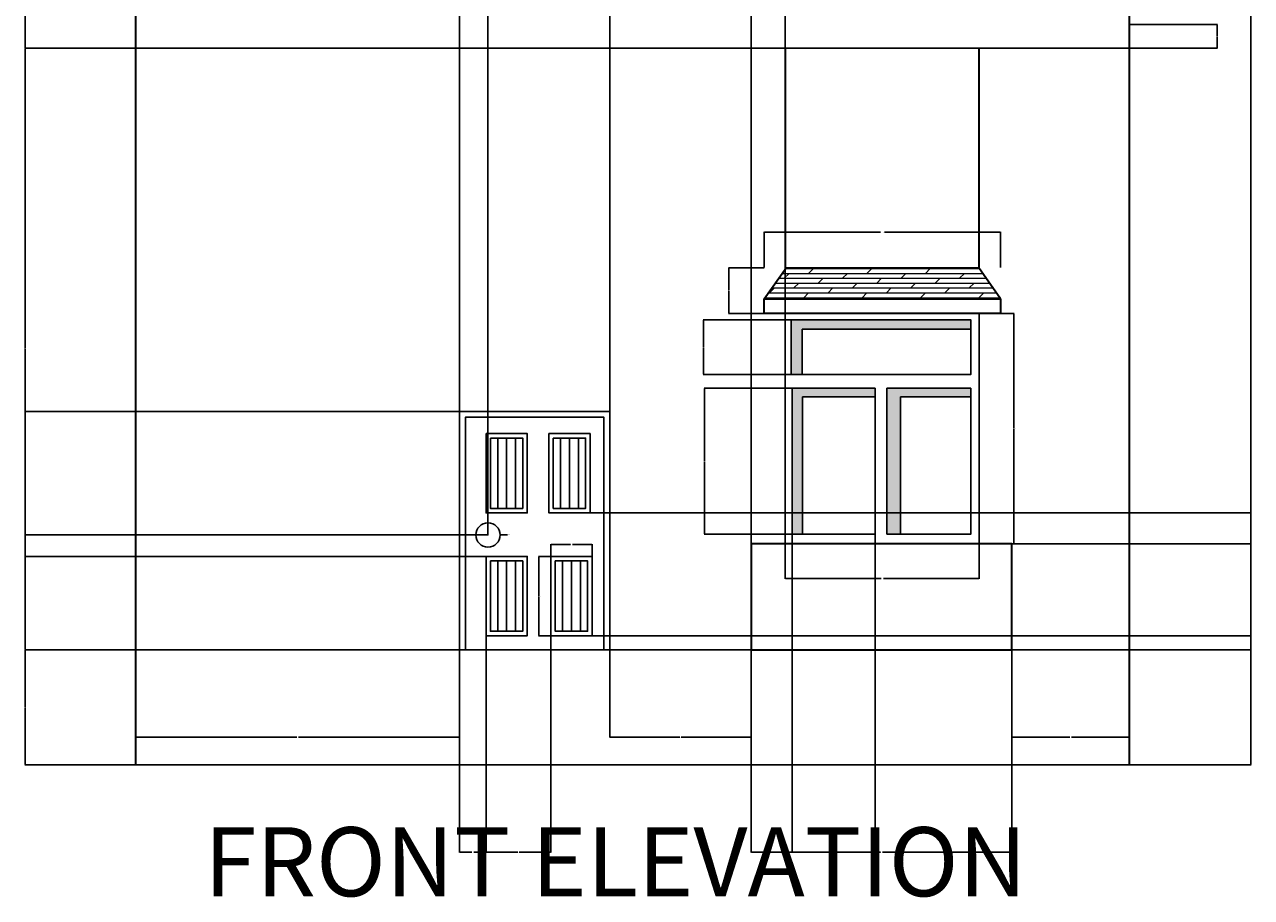
# Model space of a CAD drawing. Units: inches. Extents: x 1722 to 2362, y 1673 to 2617.
# Tile 1 of 2: x 1722 to 2362, y 1673 to 2129. Entities that reach past the tile are written whole.
import ezdxf

# ---------------------------------------------------------------- set-up
doc = ezdxf.new("R2010")
doc.units = ezdxf.units.IN
for name, color, linetype, lineweight in [('A-ANNO-DIMS', 2, 'Continuous', 18), ('A-ANNO-TEXT', 7, 'Continuous', 25), ('A-DOOR', 3, 'Continuous', 25), ('A-FLOR', 7, 'Continuous', 30), ('A-GLAZ', 4, 'Continuous', 25), ('A-GLAZ-PATT', 8, 'Continuous', 13), ('A-ROOF', 7, 'Continuous', 35), ('A-ROOF-PATT', 8, 'Continuous', 13), ('A-WALL', 7, 'Continuous', 35)]:
    doc.layers.add(name, color=color, linetype=linetype, lineweight=lineweight)
doc.styles.get("Standard").update_dxf_attribs({"font": 'arial.ttf'})
doc.dimstyles.get("Standard").update_dxf_attribs({"dimtxt": 0.18, "dimasz": 0.18, "dimexe": 0.18, "dimexo": 0.0625, "dimgap": 0.09, "dimtad": 0, "dimtih": 1, "dimtoh": 1, "dimdec": 4, "dimzin": 0, "dimdsep": 46, "dimtxsty": 'Standard', "dimcen": 0.09, "dimadec": 0, "dimazin": 0, "dimtfac": 1, "dimtdec": 4, "dimtofl": 0, "dimtmove": 0, "dimatfit": 3, "dimfxl": 1, "dimtolj": 1, "dimtzin": 0, "dimarcsym": 0})

# ---------------------------------------------------------------- blocks, each defined once
blk = doc.blocks.new('DOOR-PANEL-FLUTED')
for p, q in [((6.1, 39.03), (6.1, 2.33)), ((10.76, 39.03), (10.76, 2.33)), ((15.43, 39.03), (15.43, 2.33))]:
    blk.add_line(p, q)
for points in [[(0, 41.36), (21.52, 41.36), (21.52, 0), (0, 0)], [(2.33, 39.03), (19.19, 39.03), (19.19, 2.33), (2.33, 2.33)]]:
    blk.add_lwpolyline(points, close=True)
blk = doc.blocks.new('WIN-TWIN-TRANSOM')
for p, q in [((101.33, 120.15), (0, 120.15)), ((0, 120.15), (0, 0)), ((101.33, 0), (101.33, 120.15)), ((8.83, 88.28), (8.83, 111.99)), ((8.83, 111.99), (96.81, 111.99)), ((47.03, 81.23), (47.03, 5.04)), ((53.04, 81.23), (53.04, 5.04)), ((9.1, 76.71), (9.1, 5.04)), ((9.1, 76.71), (47.03, 76.71)), ((60.23, 76.71), (60.23, 5.04)), ((60.23, 76.71), (96.88, 76.71))]:
    blk.add_line(p, q)
blk.add_lwpolyline([(3.1, 116.89), (96.81, 116.89), (96.81, 88.28), (3.1, 88.28)], close=True)
for points in [[(47.03, 5.04), (3.67, 5.04), (3.67, 81.23), (47.03, 81.23)], [(53.04, 81.23), (96.88, 81.23), (96.88, 5.04), (53.04, 5.04)]]:
    blk.add_lwpolyline(points)
blk = doc.blocks.new('WIN-HOOD')
for p, q in [((0, 7.63), (11.4, 23.91)), ((11.4, 23.91), (111.91, 23.91)), ((123.31, 7.63), (111.91, 23.91)), ((0, 7.63), (123.31, 7.63)), ((0, 0), (0, 7.63)), ((123.31, 7.63), (123.31, 0)), ((123.31, 0), (0, 0))]:
    blk.add_line(p, q)
blk = doc.blocks.new('*D4')
at = {"layer": 'A-ANNO-DIMS', "color": 0, "lineweight": -2, "transparency": 16777216}
for p, q in [((1996.55, 1851.29), (1990.23, 1851.29)), ((1990.41, 1851.11), (1990.41, 1830.79)), ((1990.41, 1810.11), (1990.41, 1830.43)), ((1996.55, 1809.93), (1990.23, 1809.93))]:
    blk.add_line(p, q, dxfattribs=at)
at = {"layer": 'A-ANNO-DIMS', "color": 0, "transparency": 16777216}
for points in [[(1990.38, 1851.11), (1990.44, 1851.11), (1990.41, 1851.29)], [(1990.38, 1810.11), (1990.44, 1810.11), (1990.41, 1809.93)]]:
    blk.add_solid(points, dxfattribs=at)
at = {"layer": 'Defpoints', "color": 0, "transparency": 16777216}
for p in [(1990.41, 1851.29), (1996.61, 1851.29), (1996.61, 1809.93)]:
    blk.add_point(p, dxfattribs=at)
at = {"layer": 'A-ANNO-DIMS', "color": 0, "transparency": 16777216, "insert": (1990.41, 1830.61), "char_height": 0.18, "attachment_point": 5}
blk.add_mtext('\\A1;PANEL 41 TYP.', dxfattribs=at)
blk = doc.blocks.new('*D5')
at = {"layer": 'A-ANNO-DIMS', "color": 0, "lineweight": -2, "transparency": 16777216}
for p, q in [((1996.61, 1851.35), (1996.61, 1857.67)), ((1996.79, 1857.49), (2006.84, 1857.49)), ((2017.95, 1857.49), (2007.9, 1857.49)), ((2018.13, 1851.35), (2018.13, 1857.67))]:
    blk.add_line(p, q, dxfattribs=at)
at = {"layer": 'A-ANNO-DIMS', "color": 0, "transparency": 16777216}
for points in [[(1996.79, 1857.52), (1996.79, 1857.46), (1996.61, 1857.49)], [(2017.95, 1857.52), (2017.95, 1857.46), (2018.13, 1857.49)]]:
    blk.add_solid(points, dxfattribs=at)
at = {"layer": 'Defpoints', "color": 0, "transparency": 16777216}
for p in [(2018.13, 1857.49), (1996.61, 1851.29), (2018.13, 1851.29)]:
    blk.add_point(p, dxfattribs=at)
at = {"layer": 'A-ANNO-DIMS', "color": 0, "transparency": 16777216, "insert": (2007.37, 1857.49), "char_height": 0.18, "attachment_point": 5}
blk.add_mtext('\\A1;22 TYP.', dxfattribs=at)
blk = doc.blocks.new('*D6')
at = {"layer": 'A-ANNO-DIMS', "color": 0, "lineweight": -2, "transparency": 16777216}
for p, q in [((2220.22, 1977.99), (2238.36, 1977.99)), ((2238.18, 1977.81), (2238.18, 1918.1)), ((2238.18, 1858.02), (2238.18, 1917.74)), ((2220.22, 1857.84), (2238.36, 1857.84))]:
    blk.add_line(p, q, dxfattribs=at)
at = {"layer": 'A-ANNO-DIMS', "color": 0, "transparency": 16777216}
for points in [[(2238.15, 1977.81), (2238.21, 1977.81), (2238.18, 1977.99)], [(2238.15, 1858.02), (2238.21, 1858.02), (2238.18, 1857.84)]]:
    blk.add_solid(points, dxfattribs=at)
at = {"layer": 'Defpoints', "color": 0, "transparency": 16777216}
for p in [(2220.16, 1977.99), (2238.18, 1977.99), (2220.16, 1857.84)]:
    blk.add_point(p, dxfattribs=at)
at = {"layer": 'A-ANNO-DIMS', "color": 0, "transparency": 16777216, "insert": (2238.18, 1917.92), "char_height": 0.18, "attachment_point": 5}
blk.add_mtext('\\A1;WINDOW 120 TYP.', dxfattribs=at)
blk = doc.blocks.new('*D7')
at = {"layer": 'A-ANNO-DIMS', "color": 0, "lineweight": -2, "transparency": 16777216}
for p, q in [((2118.83, 1857.78), (2118.83, 1839.64)), ((2220.16, 1857.78), (2220.16, 1839.64)), ((2119.01, 1839.82), (2168.9, 1839.82)), ((2219.98, 1839.82), (2170.08, 1839.82))]:
    blk.add_line(p, q, dxfattribs=at)
at = {"layer": 'A-ANNO-DIMS', "color": 0, "transparency": 16777216}
for points in [[(2119.01, 1839.85), (2119.01, 1839.79), (2118.83, 1839.82)], [(2219.98, 1839.85), (2219.98, 1839.79), (2220.16, 1839.82)]]:
    blk.add_solid(points, dxfattribs=at)
at = {"layer": 'Defpoints', "color": 0, "transparency": 16777216}
for p in [(2118.83, 1857.84), (2220.16, 1857.84), (2220.16, 1839.82)]:
    blk.add_point(p, dxfattribs=at)
at = {"layer": 'A-ANNO-DIMS', "color": 0, "transparency": 16777216, "insert": (2169.49, 1839.82), "char_height": 0.18, "attachment_point": 5}
blk.add_mtext('\\A1;101 TYP.', dxfattribs=at)
blk = doc.blocks.new('*D8')
at = {"layer": 'A-ANNO-DIMS', "color": 0, "lineweight": -2, "transparency": 16777216}
for p, q in [((2107.97, 2001.96), (2107.97, 2020.58)), ((2108.15, 2020.4), (2168.62, 2020.4)), ((2231.1, 2020.4), (2170.63, 2020.4)), ((2231.28, 2001.96), (2231.28, 2020.58))]:
    blk.add_line(p, q, dxfattribs=at)
at = {"layer": 'A-ANNO-DIMS', "color": 0, "transparency": 16777216}
for points in [[(2108.15, 2020.43), (2108.15, 2020.37), (2107.97, 2020.4)], [(2231.1, 2020.43), (2231.1, 2020.37), (2231.28, 2020.4)]]:
    blk.add_solid(points, dxfattribs=at)
at = {"layer": 'Defpoints', "color": 0, "transparency": 16777216}
for p in [(2231.28, 2020.4), (2107.97, 2001.9), (2231.28, 2001.9)]:
    blk.add_point(p, dxfattribs=at)
at = {"layer": 'A-ANNO-DIMS', "color": 0, "transparency": 16777216, "insert": (2169.63, 2020.4), "char_height": 0.18, "attachment_point": 5}
blk.add_mtext('\\A1;HOOD 123 TYP.', dxfattribs=at)
blk = doc.blocks.new('*D9')
at = {"layer": 'A-ANNO-DIMS', "color": 0, "lineweight": -2, "transparency": 16777216}
for p, q in [((2107.91, 2001.9), (2089.3, 2001.9)), ((2089.48, 2001.72), (2089.48, 1990.13)), ((2089.48, 1978.17), (2089.48, 1989.77)), ((2107.91, 1977.99), (2089.3, 1977.99))]:
    blk.add_line(p, q, dxfattribs=at)
at = {"layer": 'A-ANNO-DIMS', "color": 0, "transparency": 16777216}
for points in [[(2089.45, 2001.72), (2089.51, 2001.72), (2089.48, 2001.9)], [(2089.45, 1978.17), (2089.51, 1978.17), (2089.48, 1977.99)]]:
    blk.add_solid(points, dxfattribs=at)
at = {"layer": 'Defpoints', "color": 0, "transparency": 16777216}
for p in [(2089.48, 2001.9), (2107.97, 2001.9), (2107.97, 1977.99)]:
    blk.add_point(p, dxfattribs=at)
at = {"layer": 'A-ANNO-DIMS', "color": 0, "transparency": 16777216, "insert": (2089.48, 1989.95), "char_height": 0.18, "attachment_point": 5}
blk.add_mtext('\\A1;24 TYP.', dxfattribs=at)
blk = doc.blocks.new('*D11')
at = {"layer": 'A-ANNO-DIMS', "color": 0, "lineweight": -2, "transparency": 16777216}
for p, q in [((2316.19, 2570.73), (2362, 2570.73)), ((2361.82, 2570.55), (2361.82, 2156.86)), ((2361.82, 1742.81), (2361.82, 2156.5)), ((2298.54, 1742.63), (2362, 1742.63))]:
    blk.add_line(p, q, dxfattribs=at)
at = {"layer": 'A-ANNO-DIMS', "color": 0, "transparency": 16777216}
for points in [[(2361.79, 2570.55), (2361.85, 2570.55), (2361.82, 2570.73)], [(2361.79, 1742.81), (2361.85, 1742.81), (2361.82, 1742.63)]]:
    blk.add_solid(points, dxfattribs=at)
at = {"layer": 'Defpoints', "color": 0, "transparency": 16777216}
for p in [(2316.12, 2570.73), (2361.82, 2570.73), (2298.48, 1742.63)]:
    blk.add_point(p, dxfattribs=at)
at = {"layer": 'A-ANNO-DIMS', "color": 0, "transparency": 16777216, "insert": (2361.82, 2156.68), "char_height": 0.18, "attachment_point": 5}
blk.add_mtext('\\A1;828.1', dxfattribs=at)
blk = doc.blocks.new('*D12')
at = {"layer": 'A-ANNO-DIMS', "color": 0, "lineweight": -2, "transparency": 16777216}
for p, q in [((1779.99, 1802.63), (1722.24, 1802.63)), ((1722.42, 1802.45), (1722.42, 1772.81)), ((1722.42, 1742.81), (1722.42, 1772.45)), ((1779.99, 1742.63), (1722.24, 1742.63))]:
    blk.add_line(p, q, dxfattribs=at)
at = {"layer": 'A-ANNO-DIMS', "color": 0, "transparency": 16777216}
for points in [[(1722.39, 1802.45), (1722.45, 1802.45), (1722.42, 1802.63)], [(1722.39, 1742.81), (1722.45, 1742.81), (1722.42, 1742.63)]]:
    blk.add_solid(points, dxfattribs=at)
at = {"layer": 'Defpoints', "color": 0, "transparency": 16777216}
for p in [(1722.42, 1802.63), (1780.05, 1802.63), (1780.05, 1742.63)]:
    blk.add_point(p, dxfattribs=at)
at = {"layer": 'A-ANNO-DIMS', "color": 0, "transparency": 16777216, "insert": (1722.42, 1772.63), "char_height": 0.18, "attachment_point": 5}
blk.add_mtext('\\A1;60', dxfattribs=at)
blk = doc.blocks.new('*D13')
at = {"layer": 'A-ANNO-DIMS', "color": 0, "lineweight": -2, "transparency": 16777216}
for p, q in [((1779.99, 2116.42), (1722.24, 2116.42)), ((1722.42, 2116.24), (1722.42, 1959.7)), ((1722.42, 1802.81), (1722.42, 1959.34)), ((1779.99, 1802.63), (1722.24, 1802.63))]:
    blk.add_line(p, q, dxfattribs=at)
at = {"layer": 'A-ANNO-DIMS', "color": 0, "transparency": 16777216}
for points in [[(1722.39, 2116.24), (1722.45, 2116.24), (1722.42, 2116.42)], [(1722.39, 1802.81), (1722.45, 1802.81), (1722.42, 1802.63)]]:
    blk.add_solid(points, dxfattribs=at)
at = {"layer": 'Defpoints', "color": 0, "transparency": 16777216}
for p in [(1722.42, 2116.42), (1780.05, 2116.42), (1780.05, 1802.63)]:
    blk.add_point(p, dxfattribs=at)
at = {"layer": 'A-ANNO-DIMS', "color": 0, "transparency": 16777216, "insert": (1722.42, 1959.52), "char_height": 0.18, "attachment_point": 5}
blk.add_mtext('\\A1;313.8', dxfattribs=at)
blk = doc.blocks.new('*D14')
at = {"layer": 'A-ANNO-DIMS', "color": 0, "lineweight": -2, "transparency": 16777216}
for p, q in [((1779.99, 2206.79), (1722.24, 2206.79)), ((1722.42, 2206.61), (1722.42, 2161.79)), ((1722.42, 2116.6), (1722.42, 2161.42)), ((1779.99, 2116.42), (1722.24, 2116.42))]:
    blk.add_line(p, q, dxfattribs=at)
at = {"layer": 'A-ANNO-DIMS', "color": 0, "transparency": 16777216}
for points in [[(1722.39, 2206.61), (1722.45, 2206.61), (1722.42, 2206.79)], [(1722.39, 2116.6), (1722.45, 2116.6), (1722.42, 2116.42)]]:
    blk.add_solid(points, dxfattribs=at)
at = {"layer": 'Defpoints', "color": 0, "transparency": 16777216}
for p in [(1722.42, 2206.79), (1780.05, 2206.79), (1780.05, 2116.42)]:
    blk.add_point(p, dxfattribs=at)
at = {"layer": 'A-ANNO-DIMS', "color": 0, "transparency": 16777216, "insert": (1722.42, 2161.6), "char_height": 0.18, "attachment_point": 5}
blk.add_mtext('\\A1;90.38', dxfattribs=at)
blk = doc.blocks.new('*D15')
at = {"layer": 'A-ANNO-DIMS', "color": 0, "lineweight": -2, "transparency": 16777216}
for p, q in [((2298.54, 2128.79), (2344.36, 2128.79)), ((2344.18, 2128.61), (2344.18, 2122.79)), ((2344.18, 2116.6), (2344.18, 2122.42)), ((2298.54, 2116.42), (2344.36, 2116.42))]:
    blk.add_line(p, q, dxfattribs=at)
at = {"layer": 'A-ANNO-DIMS', "color": 0, "transparency": 16777216}
for points in [[(2344.15, 2128.61), (2344.21, 2128.61), (2344.18, 2128.79)], [(2344.15, 2116.6), (2344.21, 2116.6), (2344.18, 2116.42)]]:
    blk.add_solid(points, dxfattribs=at)
at = {"layer": 'Defpoints', "color": 0, "transparency": 16777216}
for p in [(2298.48, 2128.79), (2298.48, 2116.42), (2344.18, 2116.42)]:
    blk.add_point(p, dxfattribs=at)
at = {"layer": 'A-ANNO-DIMS', "color": 0, "transparency": 16777216, "insert": (2344.18, 2122.6), "char_height": 0.18, "attachment_point": 5}
blk.add_mtext('\\A1;12.378', dxfattribs=at)
blk = doc.blocks.new('*D23')
at = {"layer": 'A-ANNO-DIMS', "color": 0, "lineweight": -2, "transparency": 16777216}
for p, q in [((1780.05, 1802.57), (1780.05, 1756.75)), ((1949.04, 1802.57), (1949.04, 1756.75)), ((1780.23, 1756.93), (1864.09, 1756.93)), ((1948.86, 1756.93), (1865, 1756.93))]:
    blk.add_line(p, q, dxfattribs=at)
at = {"layer": 'A-ANNO-DIMS', "color": 0, "transparency": 16777216}
for points in [[(1780.23, 1756.96), (1780.23, 1756.9), (1780.05, 1756.93)], [(1948.86, 1756.96), (1948.86, 1756.9), (1949.04, 1756.93)]]:
    blk.add_solid(points, dxfattribs=at)
at = {"layer": 'Defpoints', "color": 0, "transparency": 16777216}
for p in [(1780.05, 1802.63), (1949.04, 1802.63), (1780.05, 1756.93)]:
    blk.add_point(p, dxfattribs=at)
at = {"layer": 'A-ANNO-DIMS', "color": 0, "transparency": 16777216, "insert": (1864.55, 1756.93), "char_height": 0.18, "attachment_point": 5}
blk.add_mtext('\\A1;168.98', dxfattribs=at)
blk = doc.blocks.new('*D24')
at = {"layer": 'A-ANNO-DIMS', "color": 0, "lineweight": -2, "transparency": 16777216}
for p, q in [((2027.33, 1802.57), (2027.33, 1756.75)), ((2101.13, 1802.57), (2101.13, 1756.75)), ((2027.51, 1756.93), (2063.91, 1756.93)), ((2100.95, 1756.93), (2064.55, 1756.93))]:
    blk.add_line(p, q, dxfattribs=at)
at = {"layer": 'A-ANNO-DIMS', "color": 0, "transparency": 16777216}
for points in [[(2027.51, 1756.96), (2027.51, 1756.9), (2027.33, 1756.93)], [(2100.95, 1756.96), (2100.95, 1756.9), (2101.13, 1756.93)]]:
    blk.add_solid(points, dxfattribs=at)
at = {"layer": 'Defpoints', "color": 0, "transparency": 16777216}
for p in [(2027.33, 1802.63), (2101.13, 1802.63), (2027.33, 1756.93)]:
    blk.add_point(p, dxfattribs=at)
at = {"layer": 'A-ANNO-DIMS', "color": 0, "transparency": 16777216, "insert": (2064.23, 1756.93), "char_height": 0.18, "attachment_point": 5}
blk.add_mtext('\\A1;73.8', dxfattribs=at)
blk = doc.blocks.new('*D25')
at = {"layer": 'A-ANNO-DIMS', "color": 0, "lineweight": -2, "transparency": 16777216}
for p, q in [((2237.09, 1802.57), (2237.09, 1756.75)), ((2298.48, 1802.57), (2298.48, 1756.75)), ((2237.27, 1756.93), (2267.39, 1756.93)), ((2298.3, 1756.93), (2268.18, 1756.93))]:
    blk.add_line(p, q, dxfattribs=at)
at = {"layer": 'A-ANNO-DIMS', "color": 0, "transparency": 16777216}
for points in [[(2237.27, 1756.96), (2237.27, 1756.9), (2237.09, 1756.93)], [(2298.3, 1756.96), (2298.3, 1756.9), (2298.48, 1756.93)]]:
    blk.add_solid(points, dxfattribs=at)
at = {"layer": 'Defpoints', "color": 0, "transparency": 16777216}
for p in [(2237.09, 1802.63), (2298.48, 1802.63), (2237.09, 1756.93)]:
    blk.add_point(p, dxfattribs=at)
at = {"layer": 'A-ANNO-DIMS', "color": 0, "transparency": 16777216, "insert": (2267.78, 1756.93), "char_height": 0.18, "attachment_point": 5}
blk.add_mtext('\\A1;61.38', dxfattribs=at)
blk = doc.blocks.new('*D26')
at = {"layer": 'A-ANNO-DIMS', "color": 0, "lineweight": -2, "transparency": 16777216}
for p, q in [((1949.04, 1927.01), (1949.04, 2616.61)), ((1949.22, 2616.43), (1987.86, 2616.43)), ((2027.15, 2616.43), (1988.51, 2616.43)), ((2027.33, 1927.01), (2027.33, 2616.61))]:
    blk.add_line(p, q, dxfattribs=at)
at = {"layer": 'A-ANNO-DIMS', "color": 0, "transparency": 16777216}
for points in [[(1949.22, 2616.46), (1949.22, 2616.4), (1949.04, 2616.43)], [(2027.15, 2616.46), (2027.15, 2616.4), (2027.33, 2616.43)]]:
    blk.add_solid(points, dxfattribs=at)
at = {"layer": 'Defpoints', "color": 0, "transparency": 16777216}
for p in [(2027.33, 2616.43), (1949.04, 1926.94), (2027.33, 1926.94)]:
    blk.add_point(p, dxfattribs=at)
at = {"layer": 'A-ANNO-DIMS', "color": 0, "transparency": 16777216, "insert": (1988.18, 2616.43), "char_height": 0.18, "attachment_point": 5}
blk.add_mtext('\\A1;78.3', dxfattribs=at)
blk = doc.blocks.new('*D27')
at = {"layer": 'A-ANNO-DIMS', "color": 0, "lineweight": -2, "transparency": 16777216}
for p, q in [((1948.97, 1926.94), (1722.24, 1926.94)), ((1722.42, 1926.76), (1722.42, 1864.97)), ((1722.42, 1802.81), (1722.42, 1864.6)), ((1948.97, 1802.63), (1722.24, 1802.63))]:
    blk.add_line(p, q, dxfattribs=at)
at = {"layer": 'A-ANNO-DIMS', "color": 0, "transparency": 16777216}
for points in [[(1722.39, 1926.76), (1722.45, 1926.76), (1722.42, 1926.94)], [(1722.39, 1802.81), (1722.45, 1802.81), (1722.42, 1802.63)]]:
    blk.add_solid(points, dxfattribs=at)
at = {"layer": 'Defpoints', "color": 0, "transparency": 16777216}
for p in [(1722.42, 1926.94), (1949.04, 1926.94), (1949.04, 1802.63)]:
    blk.add_point(p, dxfattribs=at)
at = {"layer": 'A-ANNO-DIMS', "color": 0, "transparency": 16777216, "insert": (1722.42, 1864.79), "char_height": 0.18, "attachment_point": 5}
blk.add_mtext('\\A1;124.31', dxfattribs=at)
blk = doc.blocks.new('*D28')
at = {"layer": 'A-ANNO-DIMS', "color": 0, "lineweight": -2, "transparency": 16777216}
for p, q in [((1962.8, 1809.87), (1962.8, 1696.75)), ((1949.04, 1802.57), (1949.04, 1696.75)), ((1949.22, 1696.93), (1955.46, 1696.93)), ((1962.62, 1696.93), (1956.37, 1696.93))]:
    blk.add_line(p, q, dxfattribs=at)
at = {"layer": 'A-ANNO-DIMS', "color": 0, "transparency": 16777216}
for points in [[(1949.22, 1696.96), (1949.22, 1696.9), (1949.04, 1696.93)], [(1962.62, 1696.96), (1962.62, 1696.9), (1962.8, 1696.93)]]:
    blk.add_solid(points, dxfattribs=at)
at = {"layer": 'Defpoints', "color": 0, "transparency": 16777216}
for p in [(1962.8, 1809.93), (1949.04, 1802.63), (1962.8, 1696.93)]:
    blk.add_point(p, dxfattribs=at)
at = {"layer": 'A-ANNO-DIMS', "color": 0, "transparency": 16777216, "insert": (1955.92, 1696.93), "char_height": 0.18, "attachment_point": 5}
blk.add_mtext('\\A1;13.762', dxfattribs=at)
blk = doc.blocks.new('*D29')
at = {"layer": 'A-ANNO-DIMS', "color": 0, "lineweight": -2, "transparency": 16777216}
for p, q in [((1962.8, 1809.87), (1962.8, 1696.75)), ((1996.61, 1809.87), (1996.61, 1696.75)), ((1962.98, 1696.93), (1979.33, 1696.93)), ((1996.43, 1696.93), (1980.08, 1696.93))]:
    blk.add_line(p, q, dxfattribs=at)
at = {"layer": 'A-ANNO-DIMS', "color": 0, "transparency": 16777216}
for points in [[(1962.98, 1696.96), (1962.98, 1696.9), (1962.8, 1696.93)], [(1996.43, 1696.96), (1996.43, 1696.9), (1996.61, 1696.93)]]:
    blk.add_solid(points, dxfattribs=at)
at = {"layer": 'Defpoints', "color": 0, "transparency": 16777216}
for p in [(1962.8, 1809.93), (1996.61, 1809.93), (1996.61, 1696.93)]:
    blk.add_point(p, dxfattribs=at)
at = {"layer": 'A-ANNO-DIMS', "color": 0, "transparency": 16777216, "insert": (1979.7, 1696.93), "char_height": 0.18, "attachment_point": 5}
blk.add_mtext('\\A1;33.81', dxfattribs=at)
blk = doc.blocks.new('*D30')
at = {"layer": 'A-ANNO-DIMS', "color": 0, "lineweight": -2, "transparency": 16777216}
for p, q in [((2018.2, 1809.93), (2362, 1809.93)), ((2361.82, 1809.75), (2361.82, 1806.46)), ((2361.82, 1802.81), (2361.82, 1806.1)), ((2027.39, 1802.63), (2362, 1802.63))]:
    blk.add_line(p, q, dxfattribs=at)
at = {"layer": 'A-ANNO-DIMS', "color": 0, "transparency": 16777216}
for points in [[(2361.79, 1809.75), (2361.85, 1809.75), (2361.82, 1809.93)], [(2361.79, 1802.81), (2361.85, 1802.81), (2361.82, 1802.63)]]:
    blk.add_solid(points, dxfattribs=at)
at = {"layer": 'Defpoints', "color": 0, "transparency": 16777216}
for p in [(2018.13, 1809.93), (2361.82, 1809.93), (2027.33, 1802.63)]:
    blk.add_point(p, dxfattribs=at)
at = {"layer": 'A-ANNO-DIMS', "color": 0, "transparency": 16777216, "insert": (2361.82, 1806.28), "char_height": 0.18, "attachment_point": 5}
blk.add_mtext('\\A1;7.3', dxfattribs=at)
blk = doc.blocks.new('*D31')
at = {"layer": 'A-ANNO-DIMS', "color": 0, "lineweight": -2, "transparency": 16777216}
for p, q in [((2017.17, 1874.03), (2362, 1874.03)), ((2361.82, 1873.85), (2361.82, 1842.16)), ((2361.82, 1810.11), (2361.82, 1841.8)), ((2018.2, 1809.93), (2362, 1809.93))]:
    blk.add_line(p, q, dxfattribs=at)
at = {"layer": 'A-ANNO-DIMS', "color": 0, "transparency": 16777216}
for points in [[(2361.79, 1873.85), (2361.85, 1873.85), (2361.82, 1874.03)], [(2361.79, 1810.11), (2361.85, 1810.11), (2361.82, 1809.93)]]:
    blk.add_solid(points, dxfattribs=at)
at = {"layer": 'Defpoints', "color": 0, "transparency": 16777216}
for p in [(2017.11, 1874.03), (2361.82, 1874.03), (2018.13, 1809.93)]:
    blk.add_point(p, dxfattribs=at)
at = {"layer": 'A-ANNO-DIMS', "color": 0, "transparency": 16777216, "insert": (2361.82, 1841.98), "char_height": 0.18, "attachment_point": 5}
blk.add_mtext('\\A1;64.1', dxfattribs=at)
blk = doc.blocks.new('*D32')
at = {"layer": 'A-ANNO-DIMS', "color": 0, "lineweight": -2, "transparency": 16777216}
for p, q in [((1949.04, 1802.69), (1949.04, 2616.61)), ((1949.22, 2616.43), (1955.98, 2616.43)), ((1963.65, 2616.43), (1956.89, 2616.43)), ((1963.83, 1862.54), (1963.83, 2616.61))]:
    blk.add_line(p, q, dxfattribs=at)
at = {"layer": 'A-ANNO-DIMS', "color": 0, "transparency": 16777216}
for points in [[(1949.22, 2616.46), (1949.22, 2616.4), (1949.04, 2616.43)], [(1963.65, 2616.46), (1963.65, 2616.4), (1963.83, 2616.43)]]:
    blk.add_solid(points, dxfattribs=at)
at = {"layer": 'Defpoints', "color": 0, "transparency": 16777216}
for p in [(1963.83, 2616.43), (1963.83, 1862.48), (1949.04, 1802.63)]:
    blk.add_point(p, dxfattribs=at)
at = {"layer": 'A-ANNO-DIMS', "color": 0, "transparency": 16777216, "insert": (1956.43, 2616.43), "char_height": 0.18, "attachment_point": 5}
blk.add_mtext('\\A1;14.794', dxfattribs=at)
blk = doc.blocks.new('*D33')
at = {"layer": 'A-ANNO-DIMS', "color": 0, "lineweight": -2, "transparency": 16777216}
for p, q in [((1963.77, 1862.48), (1722.24, 1862.48)), ((1722.42, 1862.3), (1722.42, 1857.07)), ((1722.42, 1851.47), (1722.42, 1856.7)), ((1962.74, 1851.29), (1722.24, 1851.29))]:
    blk.add_line(p, q, dxfattribs=at)
at = {"layer": 'A-ANNO-DIMS', "color": 0, "transparency": 16777216}
for points in [[(1722.39, 1862.3), (1722.45, 1862.3), (1722.42, 1862.48)], [(1722.39, 1851.47), (1722.45, 1851.47), (1722.42, 1851.29)]]:
    blk.add_solid(points, dxfattribs=at)
at = {"layer": 'Defpoints', "color": 0, "transparency": 16777216}
for p in [(1722.42, 1862.48), (1963.83, 1862.48), (1962.8, 1851.29)]:
    blk.add_point(p, dxfattribs=at)
at = {"layer": 'A-ANNO-DIMS', "color": 0, "transparency": 16777216, "insert": (1722.42, 1856.89), "char_height": 0.18, "attachment_point": 5}
blk.add_mtext('\\A1;11.193', dxfattribs=at)
blk = doc.blocks.new('*D34')
at = {"layer": 'A-ANNO-DIMS', "color": 0, "lineweight": -2, "transparency": 16777216}
for p, q in [((2101.13, 1802.57), (2101.13, 1696.75)), ((2237.09, 1802.57), (2237.09, 1696.75)), ((2101.31, 1696.93), (2168.66, 1696.93)), ((2236.91, 1696.93), (2169.57, 1696.93))]:
    blk.add_line(p, q, dxfattribs=at)
at = {"layer": 'A-ANNO-DIMS', "color": 0, "transparency": 16777216}
for points in [[(2101.31, 1696.96), (2101.31, 1696.9), (2101.13, 1696.93)], [(2236.91, 1696.96), (2236.91, 1696.9), (2237.09, 1696.93)]]:
    blk.add_solid(points, dxfattribs=at)
at = {"layer": 'Defpoints', "color": 0, "transparency": 16777216}
for p in [(2101.13, 1802.63), (2237.09, 1802.63), (2237.09, 1696.93)]:
    blk.add_point(p, dxfattribs=at)
at = {"layer": 'A-ANNO-DIMS', "color": 0, "transparency": 16777216, "insert": (2169.11, 1696.93), "char_height": 0.18, "attachment_point": 5}
blk.add_mtext('\\A1;135.96', dxfattribs=at)
blk = doc.blocks.new('*D35')
at = {"layer": 'A-ANNO-DIMS', "color": 0, "lineweight": -2, "transparency": 16777216}
for p, q in [((2237.16, 1857.84), (2362, 1857.84)), ((2361.82, 1857.66), (2361.82, 1830.42)), ((2361.82, 1802.81), (2361.82, 1830.05)), ((2237.16, 1802.63), (2362, 1802.63))]:
    blk.add_line(p, q, dxfattribs=at)
at = {"layer": 'A-ANNO-DIMS', "color": 0, "transparency": 16777216}
for points in [[(2361.79, 1857.66), (2361.85, 1857.66), (2361.82, 1857.84)], [(2361.79, 1802.81), (2361.85, 1802.81), (2361.82, 1802.63)]]:
    blk.add_solid(points, dxfattribs=at)
at = {"layer": 'Defpoints', "color": 0, "transparency": 16777216}
for p in [(2237.09, 1857.84), (2361.82, 1857.84), (2237.09, 1802.63)]:
    blk.add_point(p, dxfattribs=at)
at = {"layer": 'A-ANNO-DIMS', "color": 0, "transparency": 16777216, "insert": (2361.82, 1830.24), "char_height": 0.18, "attachment_point": 5}
blk.add_mtext('\\A1;55.21', dxfattribs=at)
blk = doc.blocks.new('*D36')
at = {"layer": 'A-ANNO-DIMS', "color": 0, "lineweight": -2, "transparency": 16777216}
for p, q in [((2101.13, 1857.91), (2101.13, 2616.61)), ((2101.31, 2616.43), (2109.67, 2616.43)), ((2118.65, 2616.43), (2110.3, 2616.43)), ((2118.83, 1857.91), (2118.83, 2616.61))]:
    blk.add_line(p, q, dxfattribs=at)
at = {"layer": 'A-ANNO-DIMS', "color": 0, "transparency": 16777216}
for points in [[(2101.31, 2616.46), (2101.31, 2616.4), (2101.13, 2616.43)], [(2118.65, 2616.46), (2118.65, 2616.4), (2118.83, 2616.43)]]:
    blk.add_solid(points, dxfattribs=at)
at = {"layer": 'Defpoints', "color": 0, "transparency": 16777216}
for p in [(2118.83, 2616.43), (2101.13, 1857.84), (2118.83, 1857.84)]:
    blk.add_point(p, dxfattribs=at)
at = {"layer": 'A-ANNO-DIMS', "color": 0, "transparency": 16777216, "insert": (2109.98, 2616.43), "char_height": 0.18, "attachment_point": 5}
blk.add_mtext('\\A1;17.7', dxfattribs=at)
blk = doc.blocks.new('*D37')
at = {"layer": 'A-ANNO-DIMS', "color": 0, "lineweight": -2, "transparency": 16777216}
for p, q in [((2122.5, 1862.82), (2122.5, 1696.75)), ((2165.86, 1862.82), (2165.86, 1696.75)), ((2122.68, 1696.93), (2143.71, 1696.93)), ((2165.68, 1696.93), (2144.65, 1696.93))]:
    blk.add_line(p, q, dxfattribs=at)
at = {"layer": 'A-ANNO-DIMS', "color": 0, "transparency": 16777216}
for points in [[(2122.68, 1696.96), (2122.68, 1696.9), (2122.5, 1696.93)], [(2165.68, 1696.96), (2165.68, 1696.9), (2165.86, 1696.93)]]:
    blk.add_solid(points, dxfattribs=at)
at = {"layer": 'Defpoints', "color": 0, "transparency": 16777216}
for p in [(2122.5, 1862.88), (2165.86, 1862.88), (2165.86, 1696.93)]:
    blk.add_point(p, dxfattribs=at)
at = {"layer": 'A-ANNO-DIMS', "color": 0, "transparency": 16777216, "insert": (2144.18, 1696.93), "char_height": 0.18, "attachment_point": 5}
blk.add_mtext('\\A1;43.365', dxfattribs=at)
blk = doc.blocks.new('*D38')
at = {"layer": 'A-ANNO-DIMS', "color": 0, "lineweight": -2, "transparency": 16777216}
for p, q in [((2122.43, 1939.07), (2076.62, 1939.07)), ((2076.8, 1938.89), (2076.8, 1901.16)), ((2076.8, 1863.06), (2076.8, 1900.79)), ((2122.43, 1862.88), (2076.62, 1862.88))]:
    blk.add_line(p, q, dxfattribs=at)
at = {"layer": 'A-ANNO-DIMS', "color": 0, "transparency": 16777216}
for points in [[(2076.77, 1938.89), (2076.83, 1938.89), (2076.8, 1939.07)], [(2076.77, 1863.06), (2076.83, 1863.06), (2076.8, 1862.88)]]:
    blk.add_solid(points, dxfattribs=at)
at = {"layer": 'Defpoints', "color": 0, "transparency": 16777216}
for p in [(2076.8, 1939.07), (2122.5, 1939.07), (2122.5, 1862.88)]:
    blk.add_point(p, dxfattribs=at)
at = {"layer": 'A-ANNO-DIMS', "color": 0, "transparency": 16777216, "insert": (2076.8, 1900.98), "char_height": 0.18, "attachment_point": 5}
blk.add_mtext('\\A1;76.19', dxfattribs=at)
blk = doc.blocks.new('*D39')
at = {"layer": 'A-ANNO-DIMS', "color": 0, "lineweight": -2, "transparency": 16777216}
for p, q in [((2121.86, 1974.74), (2076.05, 1974.74)), ((2076.23, 1974.56), (2076.23, 1960.61)), ((2076.23, 1946.31), (2076.23, 1960.25)), ((2121.86, 1946.13), (2076.05, 1946.13))]:
    blk.add_line(p, q, dxfattribs=at)
at = {"layer": 'A-ANNO-DIMS', "color": 0, "transparency": 16777216}
for points in [[(2076.2, 1974.56), (2076.26, 1974.56), (2076.23, 1974.74)], [(2076.2, 1946.31), (2076.26, 1946.31), (2076.23, 1946.13)]]:
    blk.add_solid(points, dxfattribs=at)
at = {"layer": 'Defpoints', "color": 0, "transparency": 16777216}
for p in [(2076.23, 1974.74), (2121.93, 1974.74), (2121.93, 1946.13)]:
    blk.add_point(p, dxfattribs=at)
at = {"layer": 'A-ANNO-DIMS', "color": 0, "transparency": 16777216, "insert": (2076.23, 1960.43), "char_height": 0.18, "attachment_point": 5}
blk.add_mtext('\\A1;28.61', dxfattribs=at)
blk = doc.blocks.new('*D40')
at = {"layer": 'A-ANNO-DIMS', "color": 0, "lineweight": -2, "transparency": 16777216}
for p, q in [((1963.74, 1862.48), (1963.92, 1862.48)), ((1963.83, 1862.39), (1963.83, 1862.57)), ((1973.97, 1862.48), (1970.35, 1862.48))]:
    blk.add_line(p, q, dxfattribs=at)
at = {"layer": 'A-ANNO-DIMS', "color": 0, "transparency": 16777216}
blk.add_solid([(1970.35, 1862.51), (1970.35, 1862.45), (1970.17, 1862.48)], dxfattribs=at)
at = {"layer": 'Defpoints', "color": 0, "transparency": 16777216}
for p in [(1957.49, 1862.48), (1970.17, 1862.48)]:
    blk.add_point(p, dxfattribs=at)
at = {"layer": 'A-ANNO-DIMS', "color": 0, "transparency": 16777216, "insert": (1974.72, 1862.48), "char_height": 0.18, "attachment_point": 5}
blk.add_mtext('\\A1;2X ∅12.675', dxfattribs=at)

msp = doc.modelspace()

# ---------------------------------------------------------------- hatches: boundary and pattern name
at = {"layer": 'A-GLAZ-PATT'}
h = msp.add_hatch(color=256, dxfattribs=at)
h.dxf.hatch_style = 1
h.paths.add_polyline_path([(2127.935, 1934.5566), (2165.8618, 1934.5566), (2165.8618, 1939.0711), (2122.497, 1939.0711), (2122.497, 1862.8793), (2127.935, 1862.8793)])
h.paths.add_polyline_path([(2215.6423, 1974.7364), (2121.926, 1974.7364), (2121.926, 1946.1274), (2127.6599, 1946.1274), (2127.6599, 1969.8374), (2215.6423, 1969.8374)])
h.paths.add_polyline_path([(2179.0618, 1934.5566), (2215.7078, 1934.5566), (2215.7078, 1939.0711), (2171.8684, 1939.0711), (2171.8684, 1862.8793), (2179.0618, 1862.8793)])
h.paths.add_polyline_path([(2120.6292, 2283.5064), (2158.556, 2283.5064), (2158.556, 2288.0209), (2115.1912, 2288.0209), (2115.1912, 2211.8291), (2120.6292, 2211.8291)])
h.paths.add_polyline_path([(2171.756, 2283.5064), (2208.402, 2283.5064), (2208.402, 2288.0209), (2164.5626, 2288.0209), (2164.5626, 2211.8291), (2171.756, 2211.8291)])
h.paths.add_polyline_path([(2120.3541, 2318.7873), (2208.3365, 2318.7873), (2208.3365, 2323.6862), (2114.6202, 2323.6862), (2114.6202, 2295.0772), (2120.3541, 2295.0772)])
h = msp.add_hatch(color=256, dxfattribs=at)
h.dxf.hatch_style = 1
h.set_gradient(color1=(99, 100, 102), color2=(0, 0, 0), name='INVCYLINDER')
h.paths.add_polyline_path([(2127.935, 1934.5566), (2165.8618, 1934.5566), (2165.8618, 1939.0711), (2122.497, 1939.0711), (2122.497, 1862.8793), (2127.935, 1862.8793)])
h.paths.add_polyline_path([(2179.0618, 1934.5566), (2215.7078, 1934.5566), (2215.7078, 1939.0711), (2171.8684, 1939.0711), (2171.8684, 1862.8793), (2179.0618, 1862.8793)])
h.paths.add_polyline_path([(2127.6599, 1969.8374), (2215.6423, 1969.8374), (2215.6423, 1974.7364), (2121.926, 1974.7364), (2121.926, 1946.1274), (2127.6599, 1946.1274)])
h.paths.add_polyline_path([(2120.6292, 2283.5064), (2158.556, 2283.5064), (2158.556, 2288.0209), (2115.1912, 2288.0209), (2115.1912, 2211.8291), (2120.6292, 2211.8291)])
h.paths.add_polyline_path([(2171.756, 2283.5064), (2208.402, 2283.5064), (2208.402, 2288.0209), (2164.5626, 2288.0209), (2164.5626, 2211.8291), (2171.756, 2211.8291)])
h.paths.add_polyline_path([(2120.3541, 2318.7873), (2208.3365, 2318.7873), (2208.3365, 2323.6862), (2114.6202, 2323.6862), (2114.6202, 2295.0772), (2120.3541, 2295.0772)])
at = {"layer": 'A-ROOF-PATT'}
h = msp.add_hatch(dxfattribs=at)
h.set_pattern_fill('DOLMIT', color=256, scale=0.4)
h.paths.add_polyline_path([(2219.8784, 2001.9022), (2119.372, 2001.9022), (2107.9725, 1985.6219), (2231.2779, 1985.6219)])
h.paths.add_polyline_path([(2212.5726, 2350.8521), (2112.0662, 2350.8521), (2100.6667, 2334.5718), (2223.9721, 2334.5718)])

# ---------------------------------------------------------------- linework, layer by layer
at = {"layer": 'A-DOOR'}
for p, q in [((2027.3319, 1926.9442), (1949.0362, 1926.9442)), ((1949.0362, 1926.9442), (1949.0362, 1802.6293)), ((2027.3319, 1802.6293), (2027.3319, 1926.9442))]:
    msp.add_line(p, q, dxfattribs=at)
msp.add_lwpolyline([(1952.0362, 1802.6293), (2024.3319, 1802.6293), (2024.3319, 1923.9442), (1952.0362, 1923.9442)], close=True, dxfattribs=at)
msp.add_circle((1963.8298, 1862.4813), 6.3375, dxfattribs=at)
at = {"layer": 'A-FLOR'}
for p, q in [((1780.0546, 2116.4151), (2298.4756, 2116.4151)), ((1780.0546, 1802.6293), (2298.4756, 1802.6293)), ((1780.0546, 1742.6293), (2298.4756, 1742.6293))]:
    msp.add_line(p, q, dxfattribs=at)
at = {"layer": 'A-GLAZ'}
msp.add_line((2118.8302, 1857.8437), (2220.1562, 1857.8437), dxfattribs=at)
at = {"layer": 'A-WALL'}
for p, q in [((1780.0546, 1742.6293), (1780.0546, 2555.9811)), ((2298.4756, 1742.6293), (2298.4756, 2555.9811)), ((2118.8302, 2116.4151), (2118.8302, 2001.1284)), ((2220.1562, 2001.5054), (2220.1562, 2116.4151)), ((2237.0941, 1857.8437), (2101.1312, 1857.8437)), ((2101.1312, 1857.8437), (2101.1312, 1802.6293)), ((2237.0941, 1802.6293), (2237.0941, 1857.8437)), ((2101.1312, 1802.6293), (2237.0941, 1802.6293))]:
    msp.add_line(p, q, dxfattribs=at)

# ---------------------------------------------------------------- block references
at = {"layer": 'A-DOOR'}
for p in [(1962.798, 1874.035), (1995.583, 1874.035), (1962.798, 1809.9288), (1996.6092, 1809.9288)]:
    msp.add_blockref('DOOR-PANEL-FLUTED', p, dxfattribs=at)
at = {"layer": 'A-GLAZ'}
msp.add_blockref('WIN-TWIN-TRANSOM', (2118.83, 1857.844), dxfattribs=at)
at = {"layer": 'A-ROOF'}
msp.add_blockref('WIN-HOOD', (2107.972, 1977.995), dxfattribs=at)

# ---------------------------------------------------------------- texts
at = {"layer": 'A-ANNO-TEXT', "insert": (1815.8057, 1710.0015), "char_height": 36, "width": 532.678833, "attachment_point": 1}
msp.add_mtext('FRONT ELEVATION', dxfattribs=at)

# ---------------------------------------------------------------- dimensions: what is measured, and where the dimension line sits
at = {"layer": 'A-ANNO-DIMS'}
for base, p1, p2, override, picture, middle in [((2027.3319, 2616.4297), (1949.0362, 1926.9442), (2027.3319, 1926.9442), {"dimdec": 1, "dimlfac": 1, "dimrnd": 0, "dimzin": 0, "dimdsep": 46, "dimlunit": 2}, '*D26', (1988.1841, 2616.4297)), ((1963.8298, 2616.4297), (1949.0362, 1802.6293), (1963.8298, 1862.4813), {"dimdec": 3, "dimlfac": 1, "dimrnd": 0, "dimzin": 0, "dimdsep": 46, "dimlunit": 2}, '*D32', (1956.433, 2616.4297)), ((2118.8302, 2616.4297), (2101.1312, 1857.8437), (2118.8302, 1857.8437), {"dimdec": 1, "dimlfac": 1, "dimrnd": 0, "dimzin": 0, "dimdsep": 46, "dimlunit": 2}, '*D36', (2109.9807, 2616.4297)), ((2165.8618, 1696.9293), (2122.497, 1862.8793), (2165.8618, 1862.8793), {"dimdec": 3, "dimlfac": 1, "dimrnd": 0, "dimzin": 0, "dimdsep": 46, "dimlunit": 2}, '*D37', (2144.1794, 1696.9293)), ((1962.7979, 1696.9293), (1949.0362, 1802.6293), (1962.7979, 1809.9287), {"dimdec": 3, "dimlfac": 1, "dimrnd": 0, "dimzin": 0, "dimdsep": 46, "dimlunit": 2}, '*D28', (1955.9171, 1696.9293)), ((1996.6092, 1696.9293), (1962.7979, 1809.9287), (1996.6092, 1809.9287), {"dimdec": 2, "dimlfac": 1, "dimrnd": 0, "dimzin": 0, "dimdsep": 46, "dimlunit": 2}, '*D29', (1979.7035, 1696.9293)), ((2237.0941, 1696.9293), (2101.1312, 1802.6293), (2237.0941, 1802.6293), {"dimdec": 2, "dimlfac": 1, "dimrnd": 0, "dimzin": 0, "dimdsep": 46, "dimlunit": 2}, '*D34', (2169.1127, 1696.9293))]:
    dim = msp.add_linear_dim(base=base, p1=p1, p2=p2, dimstyle='Standard', override=override, dxfattribs=at)
    dim.commit()
    dim.dimension.update_dxf_attribs({"geometry": picture, "text_midpoint": middle})
for base, p1, p2, angle, override, picture, middle in [((2361.8231, 2570.7297), (2298.4756, 1742.6293), (2316.1231, 2570.7297), 90, {"dimdec": 1, "dimlfac": 1, "dimrnd": 0, "dimzin": 0, "dimdsep": 46, "dimlunit": 2}, '*D11', (2361.8231, 2156.6795)), ((1722.4171, 2206.7935), (1780.0546, 2116.4151), (1780.0546, 2206.7935), 90, {"dimdec": 2, "dimlfac": 1, "dimrnd": 0, "dimzin": 0, "dimdsep": 46, "dimlunit": 2}, '*D14', (1722.4171, 2161.6043)), ((2344.1756, 2116.4151), (2298.4756, 2128.7935), (2298.4756, 2116.4151), 270, {"dimdec": 3, "dimlfac": 1, "dimrnd": 0, "dimzin": 0, "dimdsep": 46, "dimlunit": 2}, '*D15', (2344.1756, 2122.6043)), ((1722.4171, 2116.4151), (1780.0546, 1802.6293), (1780.0546, 2116.4151), 90, {"dimdec": 1, "dimlfac": 1, "dimrnd": 0, "dimzin": 0, "dimdsep": 46, "dimlunit": 2}, '*D13', (1722.4171, 1959.5222)), ((2076.226, 1974.7364), (2121.926, 1946.1274), (2121.926, 1974.7364), 90, {"dimdec": 2, "dimlfac": 1, "dimrnd": 0, "dimzin": 0, "dimdsep": 46, "dimlunit": 2}, '*D39', (2076.226, 1960.4319)), ((2076.797, 1939.0711), (2122.497, 1862.8793), (2122.497, 1939.0711), 90, {"dimdec": 2, "dimlfac": 1, "dimrnd": 0, "dimzin": 0, "dimdsep": 46, "dimlunit": 2}, '*D38', (2076.797, 1900.9752)), ((1722.4171, 1926.9442), (1949.0362, 1802.6293), (1949.0362, 1926.9442), 90, {"dimdec": 2, "dimlfac": 1, "dimrnd": 0, "dimzin": 0, "dimdsep": 46, "dimlunit": 2}, '*D27', (1722.4171, 1864.7867)), ((2361.8231, 1874.0349), (2018.1328, 1809.9287), (2017.1066, 1874.0349), 90, {"dimdec": 1, "dimlfac": 1, "dimrnd": 0, "dimzin": 0, "dimdsep": 46, "dimlunit": 2}, '*D31', (2361.8231, 1841.9818)), ((1722.41713, 1862.4813), (1962.79793, 1851.28876), (1963.82983, 1862.4813), 90, {"dimdec": 3, "dimlfac": 1, "dimrnd": 0, "dimzin": 0, "dimdsep": 46, "dimlunit": 2}, '*D33', (1722.41713, 1856.88503)), ((2361.8231, 1857.8437), (2237.0941, 1802.6293), (2237.0941, 1857.8437), 90, {"dimdec": 2, "dimlfac": 1, "dimrnd": 0, "dimzin": 0, "dimdsep": 46, "dimlunit": 2}, '*D35', (2361.8231, 1830.2365)), ((2361.8231, 1809.9287), (2027.3319, 1802.6293), (2018.1328, 1809.9287), 90, {"dimdec": 1, "dimlfac": 1, "dimrnd": 0, "dimzin": 0, "dimdsep": 46, "dimlunit": 2}, '*D30', (2361.8231, 1806.279)), ((1722.4171, 1802.6293), (1780.0546, 1742.6293), (1780.0546, 1802.6293), 90, {"dimdec": 0, "dimlfac": 1, "dimrnd": 0, "dimzin": 0, "dimdsep": 46, "dimlunit": 2}, '*D12', (1722.4171, 1772.6293)), ((1780.0546, 1756.9293), (1949.0362, 1802.6293), (1780.0546, 1802.6293), 180, {"dimdec": 2, "dimlfac": 1, "dimrnd": 0, "dimzin": 0, "dimdsep": 46, "dimlunit": 2}, '*D23', (1864.5454, 1756.9293)), ((2027.3319, 1756.9293), (2101.1312, 1802.6293), (2027.3319, 1802.6293), 180, {"dimdec": 1, "dimlfac": 1, "dimrnd": 0, "dimzin": 0, "dimdsep": 46, "dimlunit": 2}, '*D24', (2064.2316, 1756.9293)), ((2237.0941, 1756.9293), (2298.4756, 1802.6293), (2237.0941, 1802.6293), 180, {"dimdec": 2, "dimlfac": 1, "dimrnd": 0, "dimzin": 0, "dimdsep": 46, "dimlunit": 2}, '*D25', (2267.7848, 1756.9293))]:
    dim = msp.add_linear_dim(base=base, p1=p1, p2=p2, angle=angle, dimstyle='Standard', override=override, dxfattribs=at)
    dim.commit()
    dim.dimension.update_dxf_attribs({"geometry": picture, "text_midpoint": middle})
for base, p1, p2, text, picture, middle in [((2231.2779, 2020.398), (2107.9725, 2001.9022), (2231.2779, 2001.9022), 'HOOD <> TYP.', '*D8', (2169.6252, 2020.398)), ((2018.1328, 1857.4928), (1996.6092, 1851.2888), (2018.1328, 1851.2888), '<> TYP.', '*D5', (2007.371, 1857.4928)), ((2220.1562, 1839.821), (2118.8302, 1857.8437), (2220.1562, 1857.8437), '<> TYP.', '*D7', (2169.4932, 1839.821))]:
    dim = msp.add_linear_dim(base=base, p1=p1, p2=p2, text=text, dimstyle='Standard', override={"dimdec": 0, "dimlfac": 1, "dimrnd": 0, "dimzin": 0, "dimdsep": 46, "dimlunit": 2}, dxfattribs=at)
    dim.commit()
    dim.dimension.update_dxf_attribs({"geometry": picture, "text_midpoint": middle})
for base, p1, p2, text, picture, middle in [((2089.4766, 2001.9022), (2107.9725, 1977.9948), (2107.9725, 2001.9022), '<> TYP.', '*D9', (2089.4766, 1989.9485)), ((2238.1789, 1977.9948), (2220.1562, 1857.8437), (2220.1562, 1977.9948), 'WINDOW <> TYP.', '*D6', (2238.1789, 1917.9193)), ((1990.4052, 1851.2888), (1996.6092, 1809.9287), (1996.6092, 1851.2888), 'PANEL <> TYP.', '*D4', (1990.4052, 1830.6088))]:
    dim = msp.add_linear_dim(base=base, p1=p1, p2=p2, angle=90, text=text, dimstyle='Standard', override={"dimdec": 0, "dimlfac": 1, "dimrnd": 0, "dimzin": 0, "dimdsep": 46, "dimlunit": 2}, dxfattribs=at)
    dim.commit()
    dim.dimension.update_dxf_attribs({"geometry": picture, "text_midpoint": middle})
dim = msp.add_diameter_dim_2p(p1=(1957.4923, 1862.4816), p2=(1970.1673, 1862.481), text='2X <>', dimstyle='Standard', override={"dimdec": 3, "dimlfac": 1, "dimrnd": 0, "dimzin": 0, "dimdsep": 46, "dimlunit": 2}, dxfattribs=at)
dim.commit()
dim.dimension.update_dxf_attribs({"geometry": '*D40', "text_midpoint": (1973.9699, 1862.4808), "dimtype": 163})

doc.saveas('drawing.dxf')
